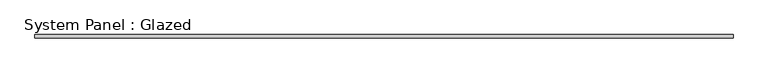
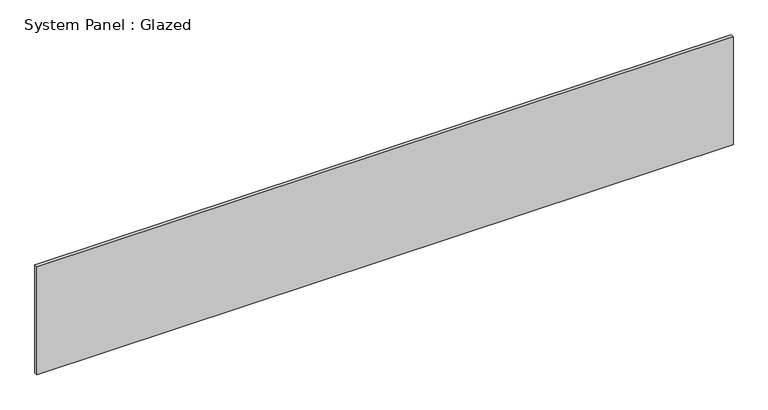
"""IFC4 building model written with IfcOpenShell, lengths in millimetres: plate geometry, System Panel : Glazed."""

from ifc_helpers import new_model, si_unit, origin, origin_with_axes, place, context, project, spatial, polyline, outline, extrude, source, transform, mapped, element, save


def system_panel_glazed_c5f16bad(model_context):
    return source(origin(), model_context, "Body", "SweptSolid", [
        extrude(outline(polyline([(2514.6, 19.05), (-2514.6, 19.05), (-2514.6, 44.45), (2514.6, 44.45), (2514.6, 19.05)])), origin_with_axes(), (0.0, 0.0, 1.0), 824.718003),
    ])


if __name__ == "__main__":
    model = new_model("IFC4")
    model_context = context("Model", 3, world=origin())
    ifc_project = project(units=[si_unit("LENGTHUNIT", "METRE", prefix="MILLI")], contexts=[model_context])
    site = spatial("IfcSite", under=ifc_project)
    building = spatial("IfcBuilding", under=site)
    placement = place(None, origin())
    system_panel_glazed_shape = system_panel_glazed_c5f16bad(model_context)
    element("IfcPlate", 1, ObjectType="System Panel : Glazed", at=placement, inside=building, context=model_context, shape_type="MappedRepresentation", body=[
        mapped(system_panel_glazed_shape, transform((0.0, 0.0, 0.0), x_axis=(1.0, 0.0, 0.0), y_axis=(0.0, 1.0, 0.0), z_axis=(0.0, 0.0, 1.0))),
    ])
    save(model, "model.ifc")

# Revit data of these elements
# Type "System Panel : Glazed"
#   Construction Type Id = "GSP4R"
#   Analytic Construction = "1/8 in Pilkington single glazing"
#   Visual Light Transmittance = 0.9
#   Solar Heat Gain Coefficient = 0.86
#   Heat Transfer Coefficient (U) = 1.18115 BTU/(h·ft²·°F)
#   Define Thermal Properties by = 1
# Element 1 (IfcPlate, "System Panel : Glazed")
#   Materials on its faces: "Glass"
# Materials
#   "Glass": class "Glass", colour RGB 0 128 192, transparency 0.75, Description = "Soda Lime Glass", Cost = 0
